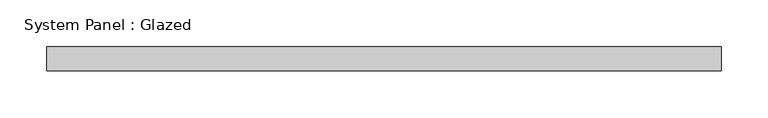
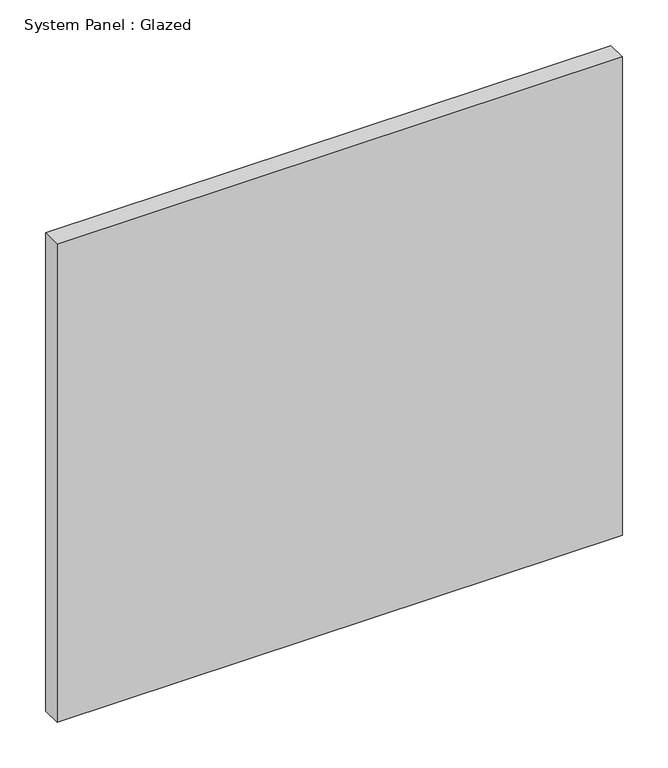
"""IFC4 building model written with IfcOpenShell, lengths in millimetres: plate geometry, System Panel : Glazed."""

from ifc_helpers import new_model, si_unit, origin, origin_with_axes, place, context, project, spatial, polyline, outline, extrude, source, transform, mapped, element, save


def system_panel_glazed_396e3693(model_context):
    return source(origin(), model_context, "Body", "SweptSolid", [
        extrude(outline(polyline([(358.775, 19.05), (-358.775, 19.05), (-358.775, 44.45), (358.775, 44.45), (358.775, 19.05)])), origin_with_axes(), (0.0, 0.0, 1.0), 641.35),
    ])


if __name__ == "__main__":
    model = new_model("IFC4")
    model_context = context("Model", 3, world=origin())
    ifc_project = project(units=[si_unit("LENGTHUNIT", "METRE", prefix="MILLI")], contexts=[model_context])
    site = spatial("IfcSite", under=ifc_project)
    building = spatial("IfcBuilding", under=site)
    placement = place(None, origin())
    system_panel_glazed_shape = system_panel_glazed_396e3693(model_context)
    element("IfcPlate", 1, ObjectType="System Panel : Glazed", at=placement, inside=building, context=model_context, shape_type="MappedRepresentation", body=[
        mapped(system_panel_glazed_shape, transform((0.0, 0.0, 0.0), x_axis=(1.0, 0.0, 0.0), y_axis=(0.0, 1.0, 0.0), z_axis=(0.0, 0.0, 1.0))),
    ])
    save(model, "model.ifc")

# Revit data of these elements
# Type "System Panel : Glazed"
#   Construction Type Id = "GSP4R"
#   Analytic Construction = "1/8 in Pilkington single glazing"
#   Visual Light Transmittance = 0.9
#   Solar Heat Gain Coefficient = 0.86
#   Heat Transfer Coefficient (U) = 1.18115 BTU/(h·ft²·°F)
#   Define Thermal Properties by = 1
# Element 1 (IfcPlate, "System Panel : Glazed")
#   Materials on its faces: "Glass"
# Materials
#   "Glass": class "Glass", colour RGB 0 128 192, transparency 0.75, Description = "Soda Lime Glass", Cost = 0
